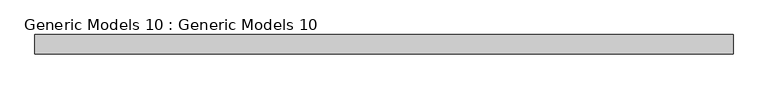
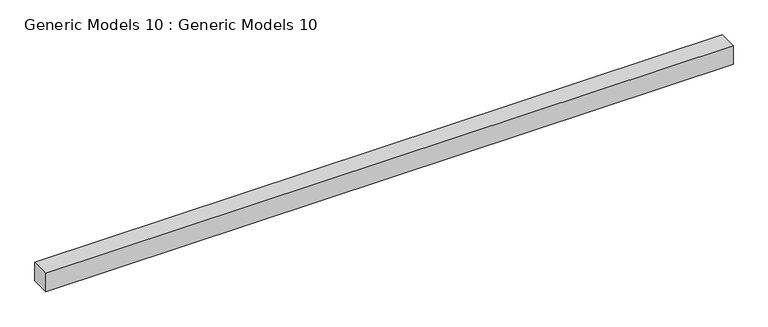
"""IFC4 building model written with IfcOpenShell, lengths in millimetres: proxy geometry, Generic Models 10 : Generic Models 10."""

from ifc_helpers import new_model, si_unit, frame, origin, place, context, project, spatial, polyline, outline, extrude, source, transform, mapped, element, save


def generic_models_10_generic_models_10_788d613d(model_context):
    return source(origin(), model_context, "Body", "SweptSolid", [
        extrude(outline(polyline([(3342.6371953, -21150.5985361), (-7701.088074, -21150.5985361), (-7701.088074, -20845.7985361), (3342.6371953, -20845.7985361), (3342.6371953, -21150.5985361)])), frame((0.0, 0.0, 9442.8162186), z_axis=(0.0, 0.0, 1.0), x_axis=(1.0, 0.0, 0.0)), (0.0, 0.0, 1.0), 310.7837814),
    ])


if __name__ == "__main__":
    model = new_model("IFC4")
    model_context = context("Model", 3, world=origin())
    ifc_project = project(units=[si_unit("LENGTHUNIT", "METRE", prefix="MILLI")], contexts=[model_context])
    site = spatial("IfcSite", under=ifc_project)
    building = spatial("IfcBuilding", under=site)
    placement = place(None, origin())
    generic_models_10_generic_models_10_shape = generic_models_10_generic_models_10_788d613d(model_context)
    element("IfcBuildingElementProxy", 1, Name="Generic Models 10 : Generic Models 10", ObjectType="Generic Models 10 : Generic Models 10", at=placement, inside=building, context=model_context, shape_type="MappedRepresentation", body=[
        mapped(generic_models_10_generic_models_10_shape, transform((0.0, 0.0, 0.0), x_axis=(1.0, 0.0, 0.0), y_axis=(0.0, 1.0, 0.0), z_axis=(0.0, 0.0, 1.0))),
    ])
    save(model, "model.ifc")
